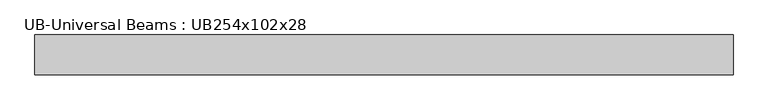
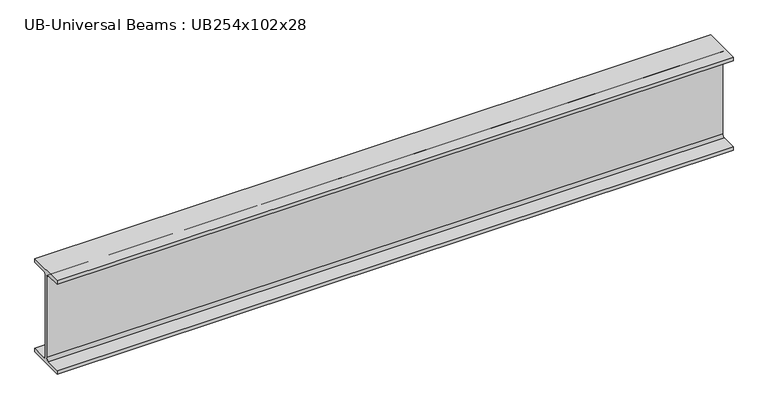
"""IFC4 building model written with IfcOpenShell, lengths in millimetres: beam geometry, UB-Universal Beams : UB254x102x28."""

from ifc_helpers import new_model, si_unit, point, frame, frame_2d, origin, place, context, project, spatial, polyline, circle_curve, trimmed, segment, composite_curve, outline, extrude, source, transform, mapped, element, save


def ub_universal_beams_ub254x102x28_a06fb1b7(model_context):
    return source(origin(), model_context, "Body", "SweptSolid", [
        extrude(outline(composite_curve([segment(polyline([(51.1, -120.2), (51.1, -130.2), (-51.1, -130.2), (-51.1, -120.2), (-10.75, -120.2)]), True, "CONTINUOUS"), segment(trimmed(circle_curve(frame_2d((-10.75, -112.6)), 7.6), [point((-10.75, -120.2))], [point((-3.15, -112.6))], True, "CARTESIAN"), True, "CONTINUOUS"), segment(polyline([(-3.15, -112.6), (-3.15, 112.6)]), True, "CONTINUOUS"), segment(trimmed(circle_curve(frame_2d((-10.75, 112.6)), 7.6), [point((-3.15, 112.6))], [point((-10.75, 120.2))], True, "CARTESIAN"), True, "CONTINUOUS"), segment(polyline([(-10.75, 120.2), (-51.1, 120.2), (-51.1, 130.2), (51.1, 130.2), (51.1, 120.2), (10.75, 120.2)]), True, "CONTINUOUS"), segment(trimmed(circle_curve(frame_2d((10.75, 112.6)), 7.6), [point((10.75, 120.2))], [point((3.15, 112.6))], True, "CARTESIAN"), True, "CONTINUOUS"), segment(polyline([(3.15, 112.6), (3.15, -112.6)]), True, "CONTINUOUS"), segment(trimmed(circle_curve(frame_2d((10.75, -112.6)), 7.6), [point((3.15, -112.6))], [point((10.75, -120.2))], True, "CARTESIAN"), True, "CONTINUOUS"), segment(polyline([(10.75, -120.2), (51.1, -120.2)]), True, "CONTINUOUS")], self_intersect=False)), frame((-1011.75, 0.0, 0.0), z_axis=(1.0, 0.0, 0.0), x_axis=(0.0, 1.0, 0.0)), (0.0, 0.0, 1.0), 1786.5),
    ])


if __name__ == "__main__":
    model = new_model("IFC4")
    model_context = context("Model", 3, world=origin())
    ifc_project = project(units=[si_unit("LENGTHUNIT", "METRE", prefix="MILLI")], contexts=[model_context])
    site = spatial("IfcSite", under=ifc_project)
    building = spatial("IfcBuilding", under=site)
    placement = place(None, origin())
    ub_universal_beams_ub254x102x28_shape = ub_universal_beams_ub254x102x28_a06fb1b7(model_context)
    element("IfcBeam", 1, ObjectType="UB-Universal Beams : UB254x102x28", at=placement, inside=building, context=model_context, shape_type="MappedRepresentation", body=[
        mapped(ub_universal_beams_ub254x102x28_shape, transform((0.0, 0.0, 0.0), x_axis=(1.0, 0.0, 0.0), y_axis=(0.0, 1.0, 0.0), z_axis=(0.0, 0.0, 1.0))),
    ])
    save(model, "model.ifc")

# Revit data of these elements
# Type "UB-Universal Beams : UB254x102x28"
#   Section Name Key = "UB254X102X28"
#   Width = 10.22 cm
#   Web Thickness = 0.63 cm
#   Web Fillet = 0.76 cm
#   Warping Constant = 28000.0 cm⁶
#   Torsional Moment of Inertia = 9.57 cm⁴
#   Section Area = 36.1 cm²
#   Plastic Modulus weak axis = 54.8 cm³
#   Plastic Modulus strong axis = 353.0 cm³
#   Nominal Weight = 28.2999 kgf/m
#   Moment of Inertia weak axis = 179.00 cm⁴
#   Moment of Inertia strong axis = 4005.00 cm⁴
#   Height = 26.04 cm
#   Flange Thickness = 1.0 cm
#   Elastic Modulus weak axis = 34.9 cm³
#   Elastic Modulus strong axis = 308.0 cm³
#   Centroid Vertical = 13.02 cm
#   Centroid Horizontal = 5.11 cm
#   Bolt Spacing = 5.4 cm
#   Length [instance default] = 4' - 11.05512"
#   Structural Material [instance default] = Metal - Steel 43-275
#   Type Comments = ""
#   Assembly Code = ""
# Element 1 (IfcBeam, "UB-Universal Beams : UB254x102x28")
#   Materials on its faces: "Metal - Steel 43-275"
# Materials
#   "Metal - Steel 43-275": class "Metal", colour RGB 247 247 247, transparency 0, Cost = 0
